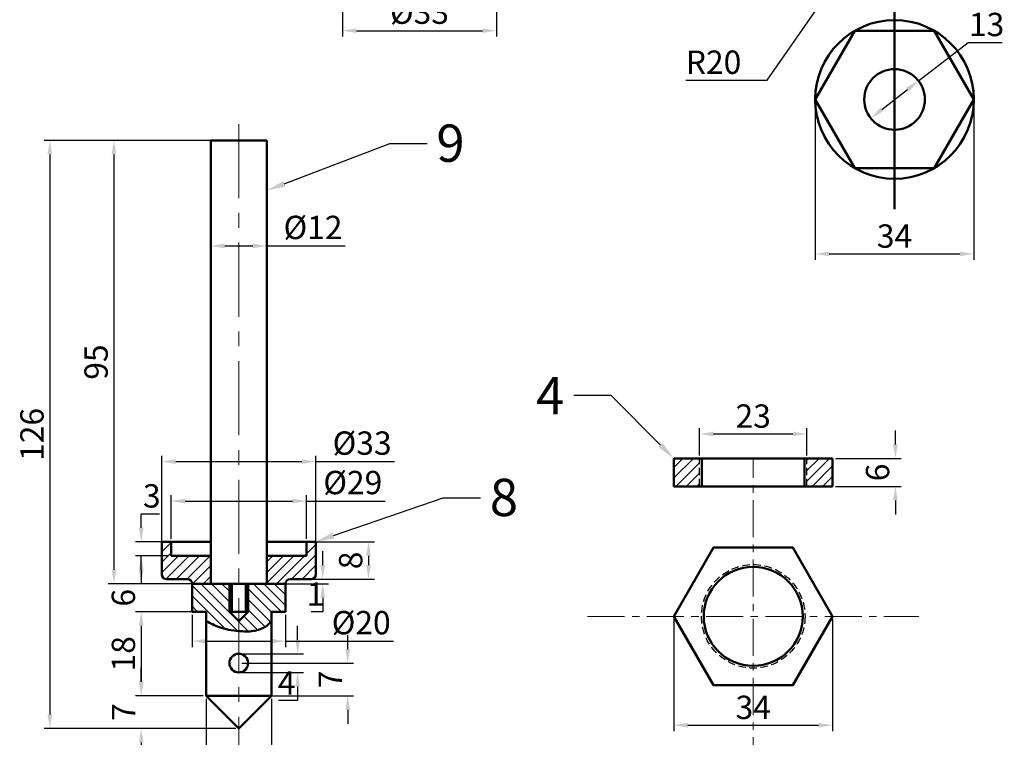
# Model space of a CAD drawing. Units: millimetres. Extents: x -656 to 85, y 134 to 571.
# Tile 3 of 5: x -393 to -182, y 281 to 435. Entities that reach past the tile are written whole.
import ezdxf
from ezdxf import colors
from ezdxf.entities.mleader import LeaderData, LeaderLine
from ezdxf.math import Vec2, Vec3

# ---------------------------------------------------------------- set-up
doc = ezdxf.new("R2010")
doc.units = ezdxf.units.MM
doc.header["$LTSCALE"] = 0.5
doc.linetypes.add('CENTER', pattern=[50.8, 31.75, -6.35, 6.35, -6.35])
doc.linetypes.add('HIDDEN', pattern=[9.525, 6.35, -3.175])
for name, color, linetype, lineweight in [('M-CNTR', 1, 'CENTER', 18), ('M-DIMS', 2, 'Continuous', 25), ('M-HATC', 8, 'Continuous', 18), ('M-HIDN', 3, 'HIDDEN', 25), ('M-OUTL', 7, 'Continuous', 50), ('M-TEXT', 7, 'Continuous', 25)]:
    doc.layers.add(name, color=color, linetype=linetype, lineweight=lineweight)
doc.styles.get("Standard").update_dxf_attribs({"font": 'arial.ttf'})
doc.dimstyles.new('ISO-25', dxfattribs={"dimtxt": 5, "dimasz": 3, "dimexe": 1.25, "dimexo": 0.625, "dimtad": 1, "dimtoh": 1, "dimdec": 0, "dimtxsty": 'Standard', "dimcen": 2.5, "dimadec": 0, "dimazin": 0, "dimtfac": 1, "dimtdec": 0, "dimtofl": 0, "dimtmove": 0, "dimatfit": 3, "dimfxl": 1, "dimarcsym": 0})

# ---------------------------------------------------------------- blocks, each defined once
blk = doc.blocks.new('*D30')
at = {"layer": 'Defpoints', "color": 0, "ltscale": 0.5, "transparency": 16777216}
for p in [(-218.5, 341.1), (-218.5, 335.1), (-205.03, 335.1)]:
    blk.add_point(p, dxfattribs=at)
at = {"layer": 'M-DIMS', "color": 0, "lineweight": -2, "ltscale": 0.5, "transparency": 16777216}
for p, q in [((-205.03, 344.1), (-205.03, 347.1)), ((-217.88, 341.1), (-203.78, 341.1)), ((-217.88, 335.1), (-203.78, 335.1)), ((-205.03, 332.1), (-205.03, 329.1))]:
    blk.add_line(p, q, dxfattribs=at)
at = {"layer": 'M-DIMS', "color": 0, "ltscale": 0.5, "transparency": 16777216}
for points in [[(-205.53, 344.1), (-204.53, 344.1), (-205.03, 341.1)], [(-205.53, 332.1), (-204.53, 332.1), (-205.03, 335.1)]]:
    blk.add_solid(points, dxfattribs=at)
at = {"layer": 'M-DIMS', "color": 0, "ltscale": 0.5, "transparency": 16777216, "insert": (-208.21, 338.1), "char_height": 5, "attachment_point": 5, "rotation": 90}
blk.add_mtext('6', dxfattribs=at)
blk = doc.blocks.new('*D31')
at = {"layer": 'Defpoints', "color": 0, "ltscale": 0.5, "transparency": 16777216}
for p in [(-252.5, 307.26), (-218.5, 307.26), (-218.5, 283.93)]:
    blk.add_point(p, dxfattribs=at)
at = {"layer": 'M-DIMS', "color": 0, "lineweight": -2, "ltscale": 0.5, "transparency": 16777216}
for p, q in [((-252.5, 306.64), (-252.5, 282.68)), ((-218.5, 306.64), (-218.5, 282.68)), ((-249.5, 283.93), (-221.5, 283.93))]:
    blk.add_line(p, q, dxfattribs=at)
at = {"layer": 'M-DIMS', "color": 0, "ltscale": 0.5, "transparency": 16777216}
for points in [[(-249.5, 284.43), (-249.5, 283.43), (-252.5, 283.93)], [(-221.5, 284.43), (-221.5, 283.43), (-218.5, 283.93)]]:
    blk.add_solid(points, dxfattribs=at)
at = {"layer": 'M-DIMS', "color": 0, "ltscale": 0.5, "transparency": 16777216, "insert": (-235.5, 287.11), "char_height": 5, "attachment_point": 5}
blk.add_mtext('34', dxfattribs=at)
blk = doc.blocks.new('*D32')
at = {"layer": 'Defpoints', "color": 0, "ltscale": 0.5, "transparency": 16777216}
for p in [(-224, 346.34), (-247, 341.1), (-224, 341.1)]:
    blk.add_point(p, dxfattribs=at)
at = {"layer": 'M-DIMS', "color": 0, "lineweight": -2, "ltscale": 0.5, "transparency": 16777216}
for p, q in [((-247, 341.72), (-247, 347.59)), ((-244, 346.34), (-227, 346.34)), ((-224, 341.72), (-224, 347.59))]:
    blk.add_line(p, q, dxfattribs=at)
at = {"layer": 'M-DIMS', "color": 0, "ltscale": 0.5, "transparency": 16777216}
for points in [[(-244, 346.84), (-244, 345.84), (-247, 346.34)], [(-227, 346.84), (-227, 345.84), (-224, 346.34)]]:
    blk.add_solid(points, dxfattribs=at)
at = {"layer": 'M-DIMS', "color": 0, "ltscale": 0.5, "transparency": 16777216, "insert": (-235.5, 349.52), "char_height": 5, "attachment_point": 5}
blk.add_mtext('23', dxfattribs=at)
blk = doc.blocks.new('*D33')
at = {"layer": 'Defpoints', "color": 0, "ltscale": 0.5, "transparency": 16777216}
for p in [(-323.49, 445.02), (-290.49, 445.02), (-290.49, 432.74)]:
    blk.add_point(p, dxfattribs=at)
at = {"layer": 'M-DIMS', "color": 0, "lineweight": -2, "ltscale": 0.5, "transparency": 16777216}
for p, q in [((-323.49, 444.4), (-323.49, 431.49)), ((-290.49, 444.4), (-290.49, 431.49)), ((-320.49, 432.74), (-293.49, 432.74))]:
    blk.add_line(p, q, dxfattribs=at)
at = {"layer": 'M-DIMS', "color": 0, "ltscale": 0.5, "transparency": 16777216}
for points in [[(-320.49, 433.24), (-320.49, 432.24), (-323.49, 432.74)], [(-293.49, 433.24), (-293.49, 432.24), (-290.49, 432.74)]]:
    blk.add_solid(points, dxfattribs=at)
at = {"layer": 'M-DIMS', "color": 0, "ltscale": 0.5, "transparency": 16777216, "insert": (-306.99, 436.06), "char_height": 5, "attachment_point": 5}
blk.add_mtext('%%C33', dxfattribs=at)
blk = doc.blocks.new('*D50')
at = {"layer": 'Defpoints', "color": 0, "ltscale": 0.5, "transparency": 16777216}
for p in [(-222.23, 418.01), (-188.23, 418.01), (-188.23, 384.91)]:
    blk.add_point(p, dxfattribs=at)
at = {"layer": 'M-DIMS', "color": 0, "lineweight": -2, "ltscale": 0.5, "transparency": 16777216}
for p, q in [((-222.23, 417.38), (-222.23, 383.66)), ((-188.23, 417.38), (-188.23, 383.66)), ((-219.23, 384.91), (-191.23, 384.91))]:
    blk.add_line(p, q, dxfattribs=at)
at = {"layer": 'M-DIMS', "color": 0, "ltscale": 0.5, "transparency": 16777216}
for points in [[(-219.23, 385.41), (-219.23, 384.41), (-222.23, 384.91)], [(-191.23, 385.41), (-191.23, 384.41), (-188.23, 384.91)]]:
    blk.add_solid(points, dxfattribs=at)
at = {"layer": 'M-DIMS', "color": 0, "ltscale": 0.5, "transparency": 16777216, "insert": (-205.23, 388.09), "char_height": 5, "attachment_point": 5}
blk.add_mtext('34', dxfattribs=at)
blk = doc.blocks.new('*D51')
at = {"layer": 'Defpoints', "color": 0, "ltscale": 0.5, "transparency": 16777216}
for p in [(-200.1, 422), (-200.08, 421.98), (-210.36, 414.02)]:
    blk.add_point(p, dxfattribs=at)
at = {"layer": 'M-DIMS', "color": 0, "lineweight": -2, "ltscale": 0.5, "transparency": 16777216}
for p, q in [((-200.08, 421.98), (-189.47, 430.24)), ((-189.47, 430.24), (-182.15, 430.24)), ((-207.97, 415.83), (-202.45, 420.13)), ((-199.72, 421.51), (-199.32, 420.99)), ((-209.98, 413.52), (-209.57, 413.01))]:
    blk.add_line(p, q, dxfattribs=at)
at = {"layer": 'M-DIMS', "color": 0, "ltscale": 0.5, "transparency": 16777216}
for points in [[(-202.76, 420.53), (-202.14, 419.74), (-200.08, 421.98)], [(-208.28, 416.23), (-207.67, 415.44), (-210.34, 413.99)]]:
    blk.add_solid(points, dxfattribs=at)
at = {"layer": 'M-DIMS', "color": 0, "ltscale": 0.5, "transparency": 16777216, "insert": (-185.5, 433.42), "char_height": 5, "attachment_point": 5}
blk.add_mtext('13', dxfattribs=at)
blk = doc.blocks.new('*D54')
at = {"layer": 'Defpoints', "color": 0, "ltscale": 0.5, "transparency": 16777216}
for p in [(-205.23, 461.18), (-216.61, 444.92)]:
    blk.add_point(p, dxfattribs=at)
at = {"layer": 'M-DIMS', "color": 0, "lineweight": -2, "ltscale": 0.5, "transparency": 16777216}
for p, q in [((-205.23, 458.68), (-205.23, 463.68)), ((-207.73, 461.18), (-202.73, 461.18)), ((-232.53, 422.16), (-218.33, 442.46)), ((-249.97, 422.16), (-232.53, 422.16))]:
    blk.add_line(p, q, dxfattribs=at)
blk.add_arc((-205.23, 461.18), 19.85, 231.4164, 235.9903, dxfattribs=at)
at = {"layer": 'M-DIMS', "color": 0, "ltscale": 0.5, "transparency": 16777216}
blk.add_solid([(-218.74, 442.75), (-217.92, 442.18), (-216.61, 444.92)], dxfattribs=at)
at = {"layer": 'M-DIMS', "color": 0, "ltscale": 0.5, "transparency": 16777216, "insert": (-244, 425.34), "char_height": 5, "attachment_point": 5}
blk.add_mtext('R20', dxfattribs=at)
blk = doc.blocks.new('*U56')
at = {"layer": 'M-CNTR', "color": 0, "transparency": 16777216}
blk.add_line((0, 51), (0, -85.46), dxfattribs=at)
blk = doc.blocks.new('*D57')
at = {"layer": 'Defpoints', "color": 0, "ltscale": 0.5, "transparency": 16777216}
for p in [(-351.71, 386.82), (-339.71, 386.82), (-339.71, 386.62)]:
    blk.add_point(p, dxfattribs=at)
at = {"layer": 'M-DIMS', "color": 0, "lineweight": -2, "ltscale": 0.5, "transparency": 16777216}
for p, q in [((-351.71, 386.2), (-351.71, 385.37)), ((-348.71, 386.62), (-342.71, 386.62)), ((-339.71, 386.62), (-322.91, 386.62)), ((-339.71, 386.2), (-339.71, 385.37))]:
    blk.add_line(p, q, dxfattribs=at)
at = {"layer": 'M-DIMS', "color": 0, "ltscale": 0.5, "transparency": 16777216}
for points in [[(-348.71, 387.12), (-348.71, 386.12), (-351.71, 386.62)], [(-342.71, 387.12), (-342.71, 386.12), (-339.71, 386.62)]]:
    blk.add_solid(points, dxfattribs=at)
at = {"layer": 'M-DIMS', "color": 0, "ltscale": 0.5, "transparency": 16777216, "insert": (-329.81, 389.94), "char_height": 5, "attachment_point": 5}
blk.add_mtext('%%C12', dxfattribs=at)
blk = doc.blocks.new('*D58')
at = {"layer": 'Defpoints', "color": 0, "ltscale": 0.5, "transparency": 16777216}
for p in [(-354.81, 314.24), (-366.6, 308.24), (-354.81, 308.24)]:
    blk.add_point(p, dxfattribs=at)
at = {"layer": 'M-DIMS', "color": 0, "lineweight": -2, "ltscale": 0.5, "transparency": 16777216}
for p, q in [((-366.6, 317.24), (-366.6, 320.24)), ((-355.44, 314.24), (-367.85, 314.24)), ((-355.44, 308.24), (-367.85, 308.24)), ((-366.6, 305.24), (-366.6, 302.24))]:
    blk.add_line(p, q, dxfattribs=at)
at = {"layer": 'M-DIMS', "color": 0, "ltscale": 0.5, "transparency": 16777216}
for points in [[(-367.1, 317.24), (-366.1, 317.24), (-366.6, 314.24)], [(-367.1, 305.24), (-366.1, 305.24), (-366.6, 308.24)]]:
    blk.add_solid(points, dxfattribs=at)
at = {"layer": 'M-DIMS', "color": 0, "ltscale": 0.5, "transparency": 16777216, "insert": (-369.78, 311.24), "char_height": 5, "attachment_point": 5, "rotation": 90}
blk.add_mtext('6', dxfattribs=at)
blk = doc.blocks.new('*D59')
at = {"layer": 'Defpoints', "color": 0, "ltscale": 0.5, "transparency": 16777216}
for p in [(-330.21, 315.24), (-336.78, 314.24), (-327.72, 314.24)]:
    blk.add_point(p, dxfattribs=at)
at = {"layer": 'M-DIMS', "color": 0, "lineweight": -2, "ltscale": 0.5, "transparency": 16777216}
for p, q in [((-327.72, 318.24), (-327.72, 321.24)), ((-329.58, 315.24), (-326.47, 315.24)), ((-336.16, 314.24), (-326.47, 314.24)), ((-327.72, 311.24), (-327.72, 308.24)), ((-327.72, 308.24), (-330.19, 308.24))]:
    blk.add_line(p, q, dxfattribs=at)
at = {"layer": 'M-DIMS', "color": 0, "ltscale": 0.5, "transparency": 16777216}
for points in [[(-328.22, 318.24), (-327.22, 318.24), (-327.72, 315.24)], [(-328.22, 311.24), (-327.22, 311.24), (-327.72, 314.24)]]:
    blk.add_solid(points, dxfattribs=at)
at = {"layer": 'M-DIMS', "color": 0, "ltscale": 0.5, "transparency": 16777216, "insert": (-329.27, 311.37), "char_height": 5, "attachment_point": 5}
blk.add_mtext('1', dxfattribs=at)
blk = doc.blocks.new('*D60')
at = {"layer": 'Defpoints', "color": 0, "ltscale": 0.5, "transparency": 16777216}
for p in [(-331.21, 323.24), (-331.21, 315.24), (-317.91, 315.24)]:
    blk.add_point(p, dxfattribs=at)
at = {"layer": 'M-DIMS', "color": 0, "lineweight": -2, "ltscale": 0.5, "transparency": 16777216}
for p, q in [((-330.58, 323.24), (-316.66, 323.24)), ((-317.91, 320.24), (-317.91, 318.24)), ((-330.58, 315.24), (-316.66, 315.24))]:
    blk.add_line(p, q, dxfattribs=at)
at = {"layer": 'M-DIMS', "color": 0, "ltscale": 0.5, "transparency": 16777216}
for points in [[(-318.41, 320.24), (-317.41, 320.24), (-317.91, 323.24)], [(-318.41, 318.24), (-317.41, 318.24), (-317.91, 315.24)]]:
    blk.add_solid(points, dxfattribs=at)
at = {"layer": 'M-DIMS', "color": 0, "ltscale": 0.5, "transparency": 16777216, "insert": (-321.09, 319.24), "char_height": 5, "attachment_point": 5, "rotation": 90}
blk.add_mtext('8', dxfattribs=at)
blk = doc.blocks.new('*D61')
at = {"layer": 'Defpoints', "color": 0, "ltscale": 0.5, "transparency": 16777216}
for p in [(-359.12, 308.24), (-366.6, 290.24), (-352.71, 290.24)]:
    blk.add_point(p, dxfattribs=at)
at = {"layer": 'M-DIMS', "color": 0, "lineweight": -2, "ltscale": 0.5, "transparency": 16777216}
for p, q in [((-359.75, 308.24), (-367.85, 308.24)), ((-366.6, 305.24), (-366.6, 293.24)), ((-353.33, 290.24), (-367.85, 290.24))]:
    blk.add_line(p, q, dxfattribs=at)
at = {"layer": 'M-DIMS', "color": 0, "ltscale": 0.5, "transparency": 16777216}
for points in [[(-367.1, 305.24), (-366.1, 305.24), (-366.6, 308.24)], [(-367.1, 293.24), (-366.1, 293.24), (-366.6, 290.24)]]:
    blk.add_solid(points, dxfattribs=at)
at = {"layer": 'M-DIMS', "color": 0, "ltscale": 0.5, "transparency": 16777216, "insert": (-369.78, 299.24), "char_height": 5, "attachment_point": 5, "rotation": 90}
blk.add_mtext('18', dxfattribs=at)
blk = doc.blocks.new('*D62')
at = {"layer": 'Defpoints', "color": 0, "ltscale": 0.5, "transparency": 16777216}
for p in [(-352.71, 290.24), (-366.6, 283.24), (-345.71, 283.24)]:
    blk.add_point(p, dxfattribs=at)
at = {"layer": 'M-DIMS', "color": 0, "lineweight": -2, "ltscale": 0.5, "transparency": 16777216}
for p, q in [((-366.6, 293.24), (-366.6, 296.24)), ((-353.33, 290.24), (-367.85, 290.24)), ((-346.33, 283.24), (-367.85, 283.24)), ((-366.6, 280.24), (-366.6, 277.24))]:
    blk.add_line(p, q, dxfattribs=at)
at = {"layer": 'M-DIMS', "color": 0, "ltscale": 0.5, "transparency": 16777216}
for points in [[(-367.1, 293.24), (-366.1, 293.24), (-366.6, 290.24)], [(-367.1, 280.24), (-366.1, 280.24), (-366.6, 283.24)]]:
    blk.add_solid(points, dxfattribs=at)
at = {"layer": 'M-DIMS', "color": 0, "ltscale": 0.5, "transparency": 16777216, "insert": (-369.73, 286.74), "char_height": 5, "attachment_point": 5, "rotation": 90}
blk.add_mtext('7', dxfattribs=at)
blk = doc.blocks.new('*D63')
at = {"layer": 'Defpoints', "color": 0, "ltscale": 0.5, "transparency": 16777216}
for p in [(-345.71, 297.24), (-345.71, 290.24), (-322.36, 290.24)]:
    blk.add_point(p, dxfattribs=at)
at = {"layer": 'M-DIMS', "color": 0, "lineweight": -2, "ltscale": 0.5, "transparency": 16777216}
for p, q in [((-322.36, 300.24), (-322.36, 303.24)), ((-345.08, 297.24), (-321.11, 297.24)), ((-345.08, 290.24), (-321.11, 290.24)), ((-322.36, 287.24), (-322.36, 284.24))]:
    blk.add_line(p, q, dxfattribs=at)
at = {"layer": 'M-DIMS', "color": 0, "ltscale": 0.5, "transparency": 16777216}
for points in [[(-322.86, 300.24), (-321.86, 300.24), (-322.36, 297.24)], [(-322.86, 287.24), (-321.86, 287.24), (-322.36, 290.24)]]:
    blk.add_solid(points, dxfattribs=at)
at = {"layer": 'M-DIMS', "color": 0, "ltscale": 0.5, "transparency": 16777216, "insert": (-325.48, 293.74), "char_height": 5, "attachment_point": 5, "rotation": 90}
blk.add_mtext('7', dxfattribs=at)
blk = doc.blocks.new('*D64')
at = {"layer": 'Defpoints', "color": 0, "ltscale": 0.5, "transparency": 16777216}
for p in [(-345.71, 299.24), (-345.71, 295.24), (-333.1, 295.24)]:
    blk.add_point(p, dxfattribs=at)
at = {"layer": 'M-DIMS', "color": 0, "lineweight": -2, "ltscale": 0.5, "transparency": 16777216}
for p, q in [((-333.1, 302.24), (-333.1, 305.24)), ((-345.08, 299.24), (-331.85, 299.24)), ((-345.08, 295.24), (-331.85, 295.24)), ((-333.1, 292.24), (-333.1, 289.24)), ((-333.1, 289.24), (-337.18, 289.24))]:
    blk.add_line(p, q, dxfattribs=at)
at = {"layer": 'M-DIMS', "color": 0, "ltscale": 0.5, "transparency": 16777216}
for points in [[(-333.6, 302.24), (-332.6, 302.24), (-333.1, 299.24)], [(-333.6, 292.24), (-332.6, 292.24), (-333.1, 295.24)]]:
    blk.add_solid(points, dxfattribs=at)
at = {"layer": 'M-DIMS', "color": 0, "ltscale": 0.5, "transparency": 16777216, "insert": (-335.45, 292.36), "char_height": 5, "attachment_point": 5}
blk.add_mtext('4', dxfattribs=at)
blk = doc.blocks.new('*D65')
at = {"layer": 'Defpoints', "color": 0, "ltscale": 0.5, "transparency": 16777216}
for p in [(-355.71, 308.24), (-335.71, 308.24), (-335.71, 301.94)]:
    blk.add_point(p, dxfattribs=at)
at = {"layer": 'M-DIMS', "color": 0, "lineweight": -2, "ltscale": 0.5, "transparency": 16777216}
for p, q in [((-355.71, 307.61), (-355.71, 300.69)), ((-335.71, 307.61), (-335.71, 300.69)), ((-352.71, 301.94), (-338.71, 301.94)), ((-335.71, 301.94), (-312.57, 301.94))]:
    blk.add_line(p, q, dxfattribs=at)
at = {"layer": 'M-DIMS', "color": 0, "ltscale": 0.5, "transparency": 16777216}
for points in [[(-352.71, 302.44), (-352.71, 301.44), (-355.71, 301.94)], [(-338.71, 302.44), (-338.71, 301.44), (-335.71, 301.94)]]:
    blk.add_solid(points, dxfattribs=at)
at = {"layer": 'M-DIMS', "color": 0, "ltscale": 0.5, "transparency": 16777216, "insert": (-319.48, 305.26), "char_height": 5, "attachment_point": 5}
blk.add_mtext('%%C20', dxfattribs=at)
blk = doc.blocks.new('*D66')
at = {"layer": 'Defpoints', "color": 0, "ltscale": 0.5, "transparency": 16777216}
for p in [(-352.71, 290.24), (-338.71, 290.24), (-338.71, 272.9)]:
    blk.add_point(p, dxfattribs=at)
at = {"layer": 'M-DIMS', "color": 0, "lineweight": -2, "ltscale": 0.5, "transparency": 16777216}
for p, q in [((-352.71, 289.61), (-352.71, 271.65)), ((-338.71, 289.61), (-338.71, 271.65)), ((-349.71, 272.9), (-341.71, 272.9))]:
    blk.add_line(p, q, dxfattribs=at)
at = {"layer": 'M-DIMS', "color": 0, "ltscale": 0.5, "transparency": 16777216}
for points in [[(-349.71, 273.4), (-349.71, 272.4), (-352.71, 272.9)], [(-341.71, 273.4), (-341.71, 272.4), (-338.71, 272.9)]]:
    blk.add_solid(points, dxfattribs=at)
at = {"layer": 'M-DIMS', "color": 0, "ltscale": 0.5, "transparency": 16777216, "insert": (-345.71, 276.22), "char_height": 5, "attachment_point": 5}
blk.add_mtext('%%C14', dxfattribs=at)
blk = doc.blocks.new('*D67')
at = {"layer": 'Defpoints', "color": 0, "ltscale": 0.5, "transparency": 16777216}
for p in [(-329.21, 340.41), (-362.21, 316.24), (-329.21, 316.24)]:
    blk.add_point(p, dxfattribs=at)
at = {"layer": 'M-DIMS', "color": 0, "lineweight": -2, "ltscale": 0.5, "transparency": 16777216}
for p, q in [((-362.21, 316.86), (-362.21, 341.66)), ((-359.21, 340.41), (-332.21, 340.41)), ((-329.21, 316.86), (-329.21, 341.66)), ((-329.21, 340.41), (-312.36, 340.41))]:
    blk.add_line(p, q, dxfattribs=at)
at = {"layer": 'M-DIMS', "color": 0, "ltscale": 0.5, "transparency": 16777216}
for points in [[(-359.21, 340.91), (-359.21, 339.91), (-362.21, 340.41)], [(-332.21, 340.91), (-332.21, 339.91), (-329.21, 340.41)]]:
    blk.add_solid(points, dxfattribs=at)
at = {"layer": 'M-DIMS', "color": 0, "ltscale": 0.5, "transparency": 16777216, "insert": (-319.28, 343.73), "char_height": 5, "attachment_point": 5}
blk.add_mtext('%%C33', dxfattribs=at)
blk = doc.blocks.new('*D68')
at = {"layer": 'Defpoints', "color": 0, "ltscale": 0.5, "transparency": 16777216}
for p in [(-331.21, 331.96), (-360.21, 323.24), (-331.21, 323.24)]:
    blk.add_point(p, dxfattribs=at)
at = {"layer": 'M-DIMS', "color": 0, "lineweight": -2, "ltscale": 0.5, "transparency": 16777216}
for p, q in [((-360.21, 323.86), (-360.21, 333.21)), ((-357.21, 331.96), (-334.21, 331.96)), ((-331.21, 323.86), (-331.21, 333.21)), ((-331.21, 331.96), (-314.35, 331.96))]:
    blk.add_line(p, q, dxfattribs=at)
at = {"layer": 'M-DIMS', "color": 0, "ltscale": 0.5, "transparency": 16777216}
for points in [[(-357.21, 332.46), (-357.21, 331.46), (-360.21, 331.96)], [(-334.21, 332.46), (-334.21, 331.46), (-331.21, 331.96)]]:
    blk.add_solid(points, dxfattribs=at)
at = {"layer": 'M-DIMS', "color": 0, "ltscale": 0.5, "transparency": 16777216, "insert": (-321.28, 335.28), "char_height": 5, "attachment_point": 5}
blk.add_mtext('%%C29', dxfattribs=at)
blk = doc.blocks.new('*D69')
at = {"layer": 'Defpoints', "color": 0, "ltscale": 0.5, "transparency": 16777216}
for p in [(-345.71, 409.24), (-386.18, 283.24), (-345.71, 283.24)]:
    blk.add_point(p, dxfattribs=at)
at = {"layer": 'M-DIMS', "color": 0, "lineweight": -2, "ltscale": 0.5, "transparency": 16777216}
for p, q in [((-346.33, 409.24), (-387.43, 409.24)), ((-386.18, 406.24), (-386.18, 286.24)), ((-346.33, 283.24), (-387.43, 283.24))]:
    blk.add_line(p, q, dxfattribs=at)
at = {"layer": 'M-DIMS', "color": 0, "ltscale": 0.5, "transparency": 16777216}
for points in [[(-386.68, 406.24), (-385.68, 406.24), (-386.18, 409.24)], [(-386.68, 286.24), (-385.68, 286.24), (-386.18, 283.24)]]:
    blk.add_solid(points, dxfattribs=at)
at = {"layer": 'M-DIMS', "color": 0, "ltscale": 0.5, "transparency": 16777216, "insert": (-389.36, 346.24), "char_height": 5, "attachment_point": 5, "rotation": 90}
blk.add_mtext('126', dxfattribs=at)
blk = doc.blocks.new('*D70')
at = {"layer": 'Defpoints', "color": 0, "ltscale": 0.5, "transparency": 16777216}
for p in [(-366.88, 409.24), (-372.45, 314.24), (-366.88, 314.24)]:
    blk.add_point(p, dxfattribs=at)
at = {"layer": 'M-DIMS', "color": 0, "lineweight": -2, "ltscale": 0.5, "transparency": 16777216}
for p, q in [((-367.51, 409.24), (-373.7, 409.24)), ((-372.45, 406.24), (-372.45, 317.24)), ((-367.51, 314.24), (-373.7, 314.24))]:
    blk.add_line(p, q, dxfattribs=at)
at = {"layer": 'M-DIMS', "color": 0, "ltscale": 0.5, "transparency": 16777216}
for points in [[(-372.95, 406.24), (-371.95, 406.24), (-372.45, 409.24)], [(-372.95, 317.24), (-371.95, 317.24), (-372.45, 314.24)]]:
    blk.add_solid(points, dxfattribs=at)
at = {"layer": 'M-DIMS', "color": 0, "ltscale": 0.5, "transparency": 16777216, "insert": (-375.63, 361.74), "char_height": 5, "attachment_point": 5, "rotation": 90}
blk.add_mtext('95', dxfattribs=at)
blk = doc.blocks.new('*D72')
at = {"layer": 'Defpoints', "color": 0, "ltscale": 0.5, "transparency": 16777216}
for p in [(-366.6, 323.24), (-360.21, 323.24), (-360.21, 320.24)]:
    blk.add_point(p, dxfattribs=at)
at = {"layer": 'M-DIMS', "color": 0, "lineweight": -2, "ltscale": 0.5, "transparency": 16777216}
for p, q in [((-366.6, 326.24), (-366.6, 329.24)), ((-366.6, 329.24), (-362.7, 329.24)), ((-360.83, 323.24), (-367.85, 323.24)), ((-360.83, 320.24), (-367.85, 320.24)), ((-366.6, 317.24), (-366.6, 314.24))]:
    blk.add_line(p, q, dxfattribs=at)
at = {"layer": 'M-DIMS', "color": 0, "ltscale": 0.5, "transparency": 16777216}
for points in [[(-367.1, 326.24), (-366.1, 326.24), (-366.6, 323.24)], [(-367.1, 317.24), (-366.1, 317.24), (-366.6, 320.24)]]:
    blk.add_solid(points, dxfattribs=at)
at = {"layer": 'M-DIMS', "color": 0, "ltscale": 0.5, "transparency": 16777216, "insert": (-364.34, 332.42), "char_height": 5, "attachment_point": 5}
blk.add_mtext('3', dxfattribs=at)

msp = doc.modelspace()

# ---------------------------------------------------------------- hatches: boundary and pattern name
at = {"layer": 'M-HATC', "ltscale": 0.5}
h = msp.add_hatch(dxfattribs=at)
h.set_pattern_fill('ANSI31', color=256, scale=0.5)
h.set_pattern_definition([(45, (-1491.849, -76.2419), (-1.122532, 1.122532), [])])
h.paths.add_polyline_path([(-247, 341.1), (-252.5, 341.1), (-252.5, 335.1), (-247, 335.1)])
h.paths.add_polyline_path([(-224, 335.1), (-218.5, 335.1), (-218.5, 341.1), (-224, 341.1)])
h = msp.add_hatch(dxfattribs=at)
h.set_pattern_fill('ANSI31', color=256, scale=0.5)
h.set_pattern_definition([(45, (-1714.0974, -236.0228), (-1.122532, 1.122532), [])])
h.paths.add_polyline_path([(-360.21, 320.24), (-360.21, 323.24), (-362.21, 323.24), (-362.21, 316.24, 0.414214), (-361.21, 315.24), (-356.71, 315.24, -0.414214), (-355.71, 314.24), (-351.71, 314.24), (-351.71, 320.24)])
h.paths.add_polyline_path([(-339.71, 320.24), (-339.71, 314.24), (-335.71, 314.24, -0.414214), (-334.71, 315.24), (-330.21, 315.24, 0.414214), (-329.21, 316.24), (-329.21, 323.24), (-331.21, 323.24), (-331.21, 320.24)])
h = msp.add_hatch(dxfattribs=at)
h.set_pattern_fill('ANSI31', color=256, scale=0.5, angle=90)
h.set_pattern_definition([(135, (-1714.0974, -236.0228), (-1.122532, -1.122532), [])])
edge = h.paths.add_edge_path()
edge.add_line((-335.71, 308.24), (-335.71, 314.24))
edge.add_line((-335.71, 314.24), (-343.71, 314.24))
edge.add_line((-343.71, 314.24), (-343.71, 308.24))
edge.add_line((-343.71, 308.24), (-345.71, 306.24))
edge.add_line((-345.71, 306.24), (-345.71, 304.12))
edge.add_spline(control_points=[(-345.71, 304.12), (-344.66, 304.02), (-342.63, 303.92), (-340.06, 304.76), (-339.05, 305.89), (-338.71, 306.28)], knot_values=[7.370812, 7.370812, 7.370812, 7.370812, 10.51527, 13.477703, 15.023307, 15.023307, 15.023307, 15.023307], degree=3, periodic=0)
edge.add_line((-338.71, 306.28), (-338.71, 308.24))
edge.add_line((-338.71, 308.24), (-335.71, 308.24))
edge = h.paths.add_edge_path()
edge.add_line((-352.71, 308.24), (-352.71, 306.26))
edge.add_spline(control_points=[(-352.71, 306.26), (-351.78, 305.78), (-349.6, 304.63), (-347.13, 304.25), (-345.71, 304.12)], knot_values=[0, 0, 0, 0, 3.113014, 7.370812, 7.370812, 7.370812, 7.370812], degree=3, periodic=0)
edge.add_line((-345.71, 304.12), (-345.71, 306.24))
edge.add_line((-345.71, 306.24), (-347.71, 308.24))
edge.add_line((-347.71, 308.24), (-347.71, 314.24))
edge.add_line((-347.71, 314.24), (-351.71, 314.24))
edge.add_line((-351.71, 314.24), (-355.71, 314.24))
edge.add_line((-355.71, 314.24), (-355.71, 308.24))
edge.add_line((-355.71, 308.24), (-352.71, 308.24))

# ---------------------------------------------------------------- linework, layer by layer
at = {"layer": 'M-CNTR', "ltscale": 0.5}
for p, q in [((-235.5, 273.42), (-235.5, 341.1)), ((-270.99, 307.26), (-200.01, 307.26))]:
    msp.add_line(p, q, dxfattribs=at)
at = {"layer": 'M-HIDN', "ltscale": 0.5}
for p, q in [((-247, 335.1), (-247, 341.1)), ((-224, 335.1), (-224, 341.1))]:
    msp.add_line(p, q, dxfattribs=at)
msp.add_circle((-235.5, 307.26), 11.1, dxfattribs=at)
at = {"layer": 'M-OUTL', "ltscale": 0.5}
for p, q in [((-205.23, 394.53), (-205.23, 504.27)), ((-351.71, 409.24), (-351.71, 314.24)), ((-339.71, 409.24), (-351.71, 409.24)), ((-339.71, 314.24), (-339.71, 409.24)), ((-252.5, 341.1), (-218.5, 341.1)), ((-252.5, 335.1), (-252.5, 341.1)), ((-246.5, 335.1), (-246.5, 341.1)), ((-224.5, 335.1), (-224.5, 341.1)), ((-218.5, 341.1), (-218.5, 335.1)), ((-218.5, 335.1), (-252.5, 335.1)), ((-362.21, 323.24), (-351.71, 323.24)), ((-362.21, 316.24), (-362.21, 323.24)), ((-360.21, 323.24), (-351.71, 323.24)), ((-360.21, 320.24), (-360.21, 323.24)), ((-339.71, 323.24), (-331.21, 323.24)), ((-339.71, 323.24), (-329.21, 323.24)), ((-331.21, 323.24), (-331.21, 320.24)), ((-329.21, 323.24), (-329.21, 316.24)), ((-351.71, 320.24), (-360.21, 320.24)), ((-331.21, 320.24), (-339.71, 320.24)), ((-356.71, 315.24), (-361.21, 315.24)), ((-330.21, 315.24), (-334.71, 315.24)), ((-351.71, 314.24), (-339.71, 314.24)), ((-347.71, 314.24), (-347.71, 308.24)), ((-343.71, 314.24), (-347.71, 314.24)), ((-347.21, 314.24), (-347.21, 308.24)), ((-344.21, 308.24), (-344.21, 314.24)), ((-343.71, 308.24), (-343.71, 314.24)), ((-352.71, 308.24), (-352.71, 290.24)), ((-347.71, 308.24), (-343.71, 308.24)), ((-347.71, 308.24), (-345.71, 306.24)), ((-343.71, 308.24), (-345.71, 306.24)), ((-338.71, 290.24), (-338.71, 308.24)), ((-352.71, 290.24), (-338.71, 290.24)), ((-345.71, 283.24), (-352.71, 290.24)), ((-345.71, 283.24), (-338.71, 290.24))]:
    msp.add_line(p, q, dxfattribs=at)
for points in [[(-188.23, 418.01), (-196.73, 432.73), (-213.73, 432.73), (-222.23, 418.01), (-213.73, 403.29), (-196.73, 403.29)], [(-218.5, 307.26), (-227, 321.98), (-244, 321.98), (-252.5, 307.26), (-244, 292.54), (-227, 292.54)]]:
    msp.add_lwpolyline(points, close=True, dxfattribs=at)
for points in [[(-355.71, 314.24), (-355.71, 308.24), (-352.71, 308.24)], [(-335.71, 314.24), (-355.71, 314.24)], [(-338.71, 308.24), (-335.71, 308.24), (-335.71, 314.24)]]:
    msp.add_lwpolyline(points, dxfattribs=at)
for centre, radius in [((-205.23, 418.01), 17), ((-205.23, 418.01), 6.5), ((-235.5, 307.26), 10.6), ((-345.71, 297.24), 2)]:
    msp.add_circle(centre, radius, dxfattribs=at)
for centre, start, end in [((-361.21, 316.24), 180, 270), ((-356.71, 314.24), 0, 90), ((-334.71, 314.24), 90, 180), ((-330.21, 316.24), 270, 0)]:
    msp.add_arc(centre, 1, start, end, dxfattribs=at)
msp.add_open_spline([(-352.71, 306.26), (-351.78, 305.78), (-349.6, 304.63), (-346.08, 304.09), (-342.63, 303.92), (-340.06, 304.76), (-339.05, 305.89), (-338.71, 306.28)], degree=3, knots=[0, 0, 0, 0, 3.113014, 7.370812, 10.51527, 13.477703, 15.023307, 15.023307, 15.023307, 15.023307], dxfattribs=at)

# ---------------------------------------------------------------- block references
at = {"layer": 'M-CNTR'}
msp.add_blockref('*U56', (-345.71, 361.74), dxfattribs=at)

# ---------------------------------------------------------------- dimensions: what is measured, and where the dimension line sits
at = {"layer": 'M-DIMS', "ltscale": 0.5}
dim = msp.add_radius_dim(center=(-205.23, 461.18), mpoint=(-216.61, 444.92), dimstyle='ISO-25', override={"dimclrd": 0, "dimclre": 0, "dimclrt": 0}, dxfattribs=at)
dim.commit()
dim.dimension.update_dxf_attribs({"geometry": '*D54', "text_midpoint": (-244, 422.16), "dimtype": 164})
for base, p1, p2, picture, middle in [((-290.49, 432.74), (-323.49, 445.02), (-290.49, 445.02), '*D33', (-306.99, 436.06)), ((-339.71, 386.62), (-351.71, 386.82), (-339.71, 386.82), '*D57', (-329.81, 389.94)), ((-338.71, 272.9), (-352.71, 290.24), (-338.71, 290.24), '*D66', (-345.71, 276.22))]:
    dim = msp.add_linear_dim(base=base, p1=p1, p2=p2, text='%%C<>', dimstyle='ISO-25', override={"dimclrd": 0, "dimclre": 0, "dimclrt": 0}, dxfattribs=at)
    dim.commit()
    dim.dimension.update_dxf_attribs({"geometry": picture, "text_midpoint": middle})
for base, p1, p2, angle, picture, middle, dimtype in [((-200.08, 421.98), (-210.36, 414.02), (-200.1, 422), 37.8956, '*D51', (-185.5, 430.24), 161), ((-327.72, 314.24), (-330.21, 315.24), (-336.78, 314.24), 90, '*D59', (-329.27, 308.24), 160), ((-322.36, 290.24), (-345.71, 297.24), (-345.71, 290.24), 90, '*D63', (-322.36, 293.74), 160)]:
    dim = msp.add_linear_dim(base=base, p1=p1, p2=p2, angle=angle, dimstyle='ISO-25', override={"dimclrd": 0, "dimclre": 0, "dimclrt": 0}, dxfattribs=at)
    dim.commit()
    dim.dimension.update_dxf_attribs({"geometry": picture, "text_midpoint": middle, "dimtype": dimtype})
for base, p1, p2, picture, middle in [((-188.23, 384.91), (-222.23, 418.01), (-188.23, 418.01), '*D50', (-205.23, 388.09)), ((-224, 346.34), (-247, 341.1), (-224, 341.1), '*D32', (-235.5, 349.52)), ((-218.5, 283.93), (-252.5, 307.26), (-218.5, 307.26), '*D31', (-235.5, 287.11))]:
    dim = msp.add_linear_dim(base=base, p1=p1, p2=p2, dimstyle='ISO-25', override={"dimclrd": 0, "dimclre": 0, "dimclrt": 0}, dxfattribs=at)
    dim.commit()
    dim.dimension.update_dxf_attribs({"geometry": picture, "text_midpoint": middle})
for base, p1, p2, picture, middle in [((-386.18, 283.24), (-345.71, 409.24), (-345.71, 283.24), '*D69', (-389.36, 346.24)), ((-372.45, 314.24), (-366.88, 409.24), (-366.88, 314.24), '*D70', (-375.63, 361.74)), ((-205.03, 335.1), (-218.5, 341.1), (-218.5, 335.1), '*D30', (-208.21, 338.1)), ((-366.6, 323.24), (-360.21, 320.24), (-360.21, 323.24), '*D72', (-364.34, 332.42)), ((-317.91, 315.24), (-331.21, 323.24), (-331.21, 315.24), '*D60', (-321.09, 319.24)), ((-366.6, 308.24), (-354.81, 314.24), (-354.81, 308.24), '*D58', (-369.78, 311.24)), ((-366.6, 290.24), (-359.12, 308.24), (-352.71, 290.24), '*D61', (-369.78, 299.24)), ((-333.1, 295.24), (-345.71, 299.24), (-345.71, 295.24), '*D64', (-335.45, 292.36)), ((-366.6, 283.24), (-352.71, 290.24), (-345.71, 283.24), '*D62', (-369.73, 286.74))]:
    dim = msp.add_linear_dim(base=base, p1=p1, p2=p2, angle=90, dimstyle='ISO-25', override={"dimclrd": 0, "dimclre": 0, "dimclrt": 0}, dxfattribs=at)
    dim.commit()
    dim.dimension.update_dxf_attribs({"geometry": picture, "text_midpoint": middle})
for base, p1, p2, picture, middle in [((-329.21, 340.41), (-362.21, 316.24), (-329.21, 316.24), '*D67', (-319.28, 340.41)), ((-331.21, 331.96), (-360.21, 323.24), (-331.21, 323.24), '*D68', (-321.28, 331.96)), ((-335.71, 301.94), (-355.71, 308.24), (-335.71, 308.24), '*D65', (-319.48, 301.94))]:
    dim = msp.add_linear_dim(base=base, p1=p1, p2=p2, text='%%C<>', dimstyle='ISO-25', override={"dimclrd": 0, "dimclre": 0, "dimclrt": 0}, dxfattribs=at)
    dim.commit()
    dim.dimension.update_dxf_attribs({"geometry": picture, "text_midpoint": middle, "dimtype": 160})

# ---------------------------------------------------------------- leaders
at = {"layer": 'M-TEXT', "ltscale": 0.5}
ml = msp.add_multileader_mtext('Standard', dxfattribs=at)
ml.set_content('9', color=256)
ml.set_leader_properties()
ml.build(insert=Vec2(0, 0))
ctx = ml.context
ctx.base_point, ctx.char_height, ctx.plane_origin = Vec3(-305.38, 408.57), 8, Vec3(-339.71, 398.49)
notes = []
notes.append((ctx, [(0, (1, 1, 0), (-313.38, 408.57), (1, 0), 8, [(0, [(-339.71, 398.49)], 0, [])])]))
ctx.mtext.insert, ctx.mtext.flow_direction = Vec3(-303.38, 412.64), 5
ml = msp.add_multileader_mtext('Standard', dxfattribs=at)
ml.set_content('4', color=256)
ml.set_leader_properties()
ml.build(insert=Vec2(0, 0))
ctx = ml.context
ctx.base_point, ctx.char_height, ctx.plane_origin = Vec3(-283.49, 354.55), 8, Vec3(-252.5, 341.1)
ctx.text_align_type = 2
notes.append((ctx, [(0, (1, 1, 0), (-265.96, 354.55), (-1, 0), 8, [(0, [(-252.5, 341.1)], 0, [])])]))
ctx.mtext.insert, ctx.mtext.alignment, ctx.mtext.flow_direction = Vec3(-275.96, 358.55), 3, 5
ml = msp.add_multileader_mtext('Standard', dxfattribs=at)
ml.set_content('8', color=256)
ml.set_leader_properties()
ml.build(insert=Vec2(0, 0))
ctx = ml.context
ctx.base_point, ctx.char_height, ctx.plane_origin = Vec3(-293.93, 332.67), 8, Vec3(-329.21, 323.24)
notes.append((ctx, [(0, (1, 1, 0), (-301.93, 332.67), (1, 0), 8, [(0, [(-329.21, 323.24)], 0, [])])]))
ctx.mtext.insert, ctx.mtext.flow_direction = Vec3(-291.93, 336.74), 5
for ctx, leaders in notes:
    for number, flags, end, landing, length, lines in leaders:
        leader = LeaderData()
        leader.index, (leader.has_last_leader_line, leader.has_dogleg_vector, leader.attachment_direction) = number, flags
        leader.last_leader_point, leader.dogleg_vector, leader.dogleg_length = Vec3(end), Vec3(landing), length
        for number, points, colour, breaks in lines:
            line = LeaderLine()
            line.index, line.vertices, line.color, line.breaks = number, Vec3.list(points), colors.encode_raw_color(colour), breaks
            leader.lines.append(line)
        ctx.leaders.append(leader)

doc.saveas('drawing.dxf')
